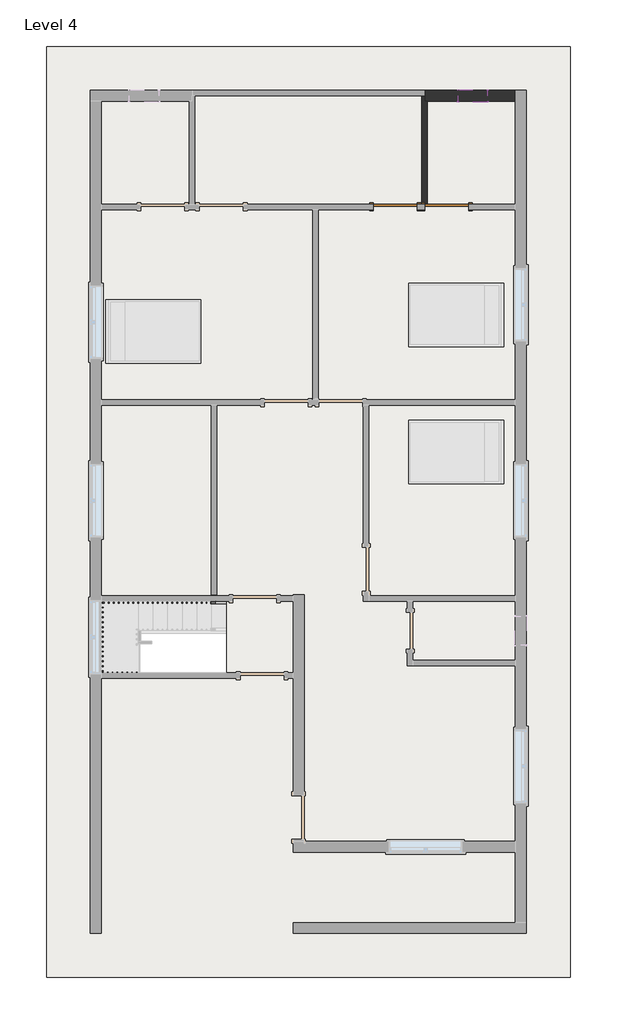
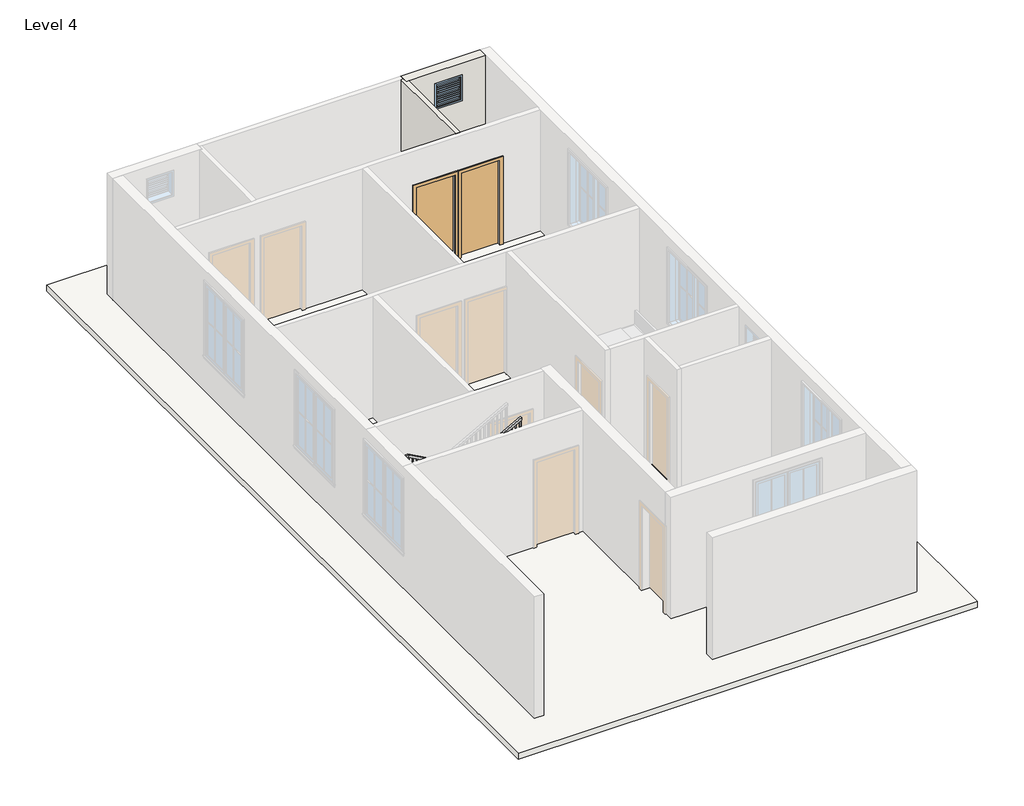
# One storey, part 2 of 3: 2 doors, 2 walls, 1 railing, 1 roof, 1 window.
"""IFC4 building model written with IfcOpenShell, lengths in millimetres."""

from ifc_helpers import new_model, si_unit, frame, origin, place, context, project, spatial, polyline, outline, extrude, faceted_brep, transform, mapped, element, save
from components import single_flush_door_3_e5f9f3c4, single_flush_door_3_305aa2a5, window_f2d8fef0

model = new_model("IFC4")

# Units and contexts
model_context = context("Model", 3, world=origin())
ifc_project = project(units=[si_unit("LENGTHUNIT", "METRE", prefix="MILLI")], contexts=[model_context])

# Site, building, storey
site = spatial("IfcSite", under=ifc_project)
building = spatial("IfcBuilding", under=site)
storey = spatial("IfcBuildingStorey", under=building, Name="Level 4", Elevation=6400.8)

# Doors
placement = place(None, origin())
single_flush_door_3_shape = single_flush_door_3_e5f9f3c4(model_context)
element("IfcDoor", 1, ObjectType="Single-Flush : DOOR 3'", at=placement, inside=storey, context=model_context, shape_type="MappedRepresentation", body=[
    mapped(single_flush_door_3_shape, transform((555.4379845, 6040.5434309, 6400.8), x_axis=(1.0, 0.0, 0.0), y_axis=(0.0, 1.0, 0.0), z_axis=(0.0, 0.0, 1.0))),
])
single_flush_door_3_2_shape = single_flush_door_3_305aa2a5(model_context)
element("IfcDoor", 2, ObjectType="Single-Flush : DOOR 3'", at=placement, inside=storey, context=model_context, shape_type="MappedRepresentation", body=[
    mapped(single_flush_door_3_2_shape, transform((1622.2379845, 6040.5434309, 6400.8), x_axis=(-1.0, 0.0, 0.0), y_axis=(0.0, -1.0, 0.0), z_axis=(0.0, 0.0, 1.0))),
])

# Railing
element("IfcRailing", 3, ObjectType="Handrail - Rectangular", at=placement, inside=storey, context=model_context, shape_type="SolidModel", body=[
    faceted_brep([(-2968.8120155, -2220.8065691, 7484.5333333), (-2968.8120155, -2220.8065691, 7426.420221), (-2968.8120155, -2170.0065691, 7426.420221), (-2968.8120155, -2170.0065691, 7484.5333333), (-4797.6120155, -2220.8065691, 8500.5333333), (-4810.7756177, -2220.8065691, 8449.7333333), (-4810.7756177, -2170.0065691, 8449.7333333), (-4797.6120155, -2170.0065691, 8500.5333333), (-5508.8120155, -2220.8065691, 8500.5333333), (-5508.8120155, -2220.8065691, 8449.7333333), (-5559.6120155, -2170.0065691, 8449.7333333), (-5559.6120155, -2170.0065691, 8500.5333333), (-5508.8120155, -3624.1565691, 8500.5333333), (-5508.8120155, -3624.1565691, 8449.7333333), (-5559.6120155, -3674.9565691, 8449.7333333), (-5559.6120155, -3674.9565691, 8500.5333333), (-5102.4120155, -3624.1565691, 8500.5333333), (-5089.2484132, -3624.1565691, 8449.7333333), (-5089.2484132, -3674.9565691, 8449.7333333), (-5102.4120155, -3674.9565691, 8500.5333333), (-2968.8120155, -3624.1565691, 9685.8666667), (-2968.8120155, -3674.9565691, 9685.8666667), (-2968.8120155, -3674.9565691, 9627.7535543), (-2968.8120155, -3624.1565691, 9627.7535543)], [[[0, 1, 2, 3]], [[1, 0, 4, 5]], [[2, 1, 5, 6]], [[3, 2, 6, 7]], [[0, 3, 7, 4]], [[5, 4, 8, 9]], [[6, 5, 9, 10]], [[7, 6, 10, 11]], [[4, 7, 11, 8]], [[9, 8, 12, 13]], [[10, 9, 13, 14]], [[11, 10, 14, 15]], [[8, 11, 15, 12]], [[13, 12, 16, 17]], [[14, 13, 17, 18]], [[15, 14, 18, 19]], [[12, 15, 19, 16]], [[20, 21, 22, 23]], [[17, 16, 20, 23]], [[18, 17, 23, 22]], [[19, 18, 22, 21]], [[16, 19, 21, 20]]]),
    extrude(outline(polyline([(9618.9341099, -2984.6870155), (9608.3507765, -3003.7370155), (8602.1333333, -3003.7370155), (8602.1333333, -2984.6870155), (9618.9341099, -2984.6870155)])), frame((0.0, -3659.0815691, 0.0), z_axis=(0.0, 1.0, 0.0), x_axis=(0.0, 0.0, 1.0)), (0.0, 0.0, 1.0), 19.05),
    extrude(outline(polyline([(9562.4896654, -3086.2870155), (9551.9063321, -3105.3370155), (8602.1333333, -3105.3370155), (8602.1333333, -3086.2870155), (9562.4896654, -3086.2870155)])), frame((0.0, -3659.0815691, 0.0), z_axis=(0.0, 1.0, 0.0), x_axis=(0.0, 0.0, 1.0)), (0.0, 0.0, 1.0), 19.05),
    extrude(outline(polyline([(9506.045221, -3187.8870155), (9495.4618876, -3206.9370155), (8602.1333333, -3206.9370155), (8602.1333333, -3187.8870155), (9506.045221, -3187.8870155)])), frame((0.0, -3659.0815691, 0.0), z_axis=(0.0, 1.0, 0.0), x_axis=(0.0, 0.0, 1.0)), (0.0, 0.0, 1.0), 19.05),
    extrude(outline(polyline([(9449.6007765, -3289.4870155), (9439.0174432, -3308.5370155), (8432.8, -3308.5370155), (8432.8, -3289.4870155), (9449.6007765, -3289.4870155)])), frame((0.0, -3659.0815691, 0.0), z_axis=(0.0, 1.0, 0.0), x_axis=(0.0, 0.0, 1.0)), (0.0, 0.0, 1.0), 19.05),
    extrude(outline(polyline([(9393.1563321, -3391.0870155), (9382.5729988, -3410.1370155), (8432.8, -3410.1370155), (8432.8, -3391.0870155), (9393.1563321, -3391.0870155)])), frame((0.0, -3659.0815691, 0.0), z_axis=(0.0, 1.0, 0.0), x_axis=(0.0, 0.0, 1.0)), (0.0, 0.0, 1.0), 19.05),
    extrude(outline(polyline([(9336.7118876, -3492.6870155), (9326.1285543, -3511.7370155), (8432.8, -3511.7370155), (8432.8, -3492.6870155), (9336.7118876, -3492.6870155)])), frame((0.0, -3659.0815691, 0.0), z_axis=(0.0, 1.0, 0.0), x_axis=(0.0, 0.0, 1.0)), (0.0, 0.0, 1.0), 19.05),
    extrude(outline(polyline([(9280.2674432, -3594.2870155), (9269.6841099, -3613.3370155), (8263.4666667, -3613.3370155), (8263.4666667, -3594.2870155), (9280.2674432, -3594.2870155)])), frame((0.0, -3659.0815691, 0.0), z_axis=(0.0, 1.0, 0.0), x_axis=(0.0, 0.0, 1.0)), (0.0, 0.0, 1.0), 19.05),
    extrude(outline(polyline([(9223.8229988, -3695.8870155), (9213.2396654, -3714.9370155), (8263.4666667, -3714.9370155), (8263.4666667, -3695.8870155), (9223.8229988, -3695.8870155)])), frame((0.0, -3659.0815691, 0.0), z_axis=(0.0, 1.0, 0.0), x_axis=(0.0, 0.0, 1.0)), (0.0, 0.0, 1.0), 19.05),
    extrude(outline(polyline([(9167.3785543, -3797.4870155), (9156.795221, -3816.5370155), (8263.4666667, -3816.5370155), (8263.4666667, -3797.4870155), (9167.3785543, -3797.4870155)])), frame((0.0, -3659.0815691, 0.0), z_axis=(0.0, 1.0, 0.0), x_axis=(0.0, 0.0, 1.0)), (0.0, 0.0, 1.0), 19.05),
    extrude(outline(polyline([(9110.9341099, -3899.0870155), (9100.3507765, -3918.1370155), (8094.1333333, -3918.1370155), (8094.1333333, -3899.0870155), (9110.9341099, -3899.0870155)])), frame((0.0, -3659.0815691, 0.0), z_axis=(0.0, 1.0, 0.0), x_axis=(0.0, 0.0, 1.0)), (0.0, 0.0, 1.0), 19.05),
    extrude(outline(polyline([(9054.4896654, -4000.6870155), (9043.9063321, -4019.7370155), (8094.1333333, -4019.7370155), (8094.1333333, -4000.6870155), (9054.4896654, -4000.6870155)])), frame((0.0, -3659.0815691, 0.0), z_axis=(0.0, 1.0, 0.0), x_axis=(0.0, 0.0, 1.0)), (0.0, 0.0, 1.0), 19.05),
    extrude(outline(polyline([(8998.045221, -4102.2870155), (8987.4618876, -4121.3370155), (8094.1333333, -4121.3370155), (8094.1333333, -4102.2870155), (8998.045221, -4102.2870155)])), frame((0.0, -3659.0815691, 0.0), z_axis=(0.0, 1.0, 0.0), x_axis=(0.0, 0.0, 1.0)), (0.0, 0.0, 1.0), 19.05),
    extrude(outline(polyline([(8941.6007765, -4203.8870155), (8931.0174432, -4222.9370155), (7924.8, -4222.9370155), (7924.8, -4203.8870155), (8941.6007765, -4203.8870155)])), frame((0.0, -3659.0815691, 0.0), z_axis=(0.0, 1.0, 0.0), x_axis=(0.0, 0.0, 1.0)), (0.0, 0.0, 1.0), 19.05),
    extrude(outline(polyline([(8885.1563321, -4305.4870155), (8874.5729988, -4324.5370155), (7924.8, -4324.5370155), (7924.8, -4305.4870155), (8885.1563321, -4305.4870155)])), frame((0.0, -3659.0815691, 0.0), z_axis=(0.0, 1.0, 0.0), x_axis=(0.0, 0.0, 1.0)), (0.0, 0.0, 1.0), 19.05),
    extrude(outline(polyline([(8828.7118876, -4407.0870155), (8818.1285543, -4426.1370155), (7924.8, -4426.1370155), (7924.8, -4407.0870155), (8828.7118876, -4407.0870155)])), frame((0.0, -3659.0815691, 0.0), z_axis=(0.0, 1.0, 0.0), x_axis=(0.0, 0.0, 1.0)), (0.0, 0.0, 1.0), 19.05),
    extrude(outline(polyline([(8772.2674432, -4508.6870155), (8761.6841099, -4527.7370155), (7755.4666667, -4527.7370155), (7755.4666667, -4508.6870155), (8772.2674432, -4508.6870155)])), frame((0.0, -3659.0815691, 0.0), z_axis=(0.0, 1.0, 0.0), x_axis=(0.0, 0.0, 1.0)), (0.0, 0.0, 1.0), 19.05),
    extrude(outline(polyline([(8715.8229988, -4610.2870155), (8705.2396654, -4629.3370155), (7755.4666667, -4629.3370155), (7755.4666667, -4610.2870155), (8715.8229988, -4610.2870155)])), frame((0.0, -3659.0815691, 0.0), z_axis=(0.0, 1.0, 0.0), x_axis=(0.0, 0.0, 1.0)), (0.0, 0.0, 1.0), 19.05),
    extrude(outline(polyline([(8659.3785543, -4711.8870155), (8648.795221, -4730.9370155), (7755.4666667, -4730.9370155), (7755.4666667, -4711.8870155), (8659.3785543, -4711.8870155)])), frame((0.0, -3659.0815691, 0.0), z_axis=(0.0, 1.0, 0.0), x_axis=(0.0, 0.0, 1.0)), (0.0, 0.0, 1.0), 19.05),
    extrude(outline(polyline([(8602.9341099, -4813.4870155), (8592.3507765, -4832.5370155), (7586.1333333, -4832.5370155), (7586.1333333, -4813.4870155), (8602.9341099, -4813.4870155)])), frame((0.0, -3659.0815691, 0.0), z_axis=(0.0, 1.0, 0.0), x_axis=(0.0, 0.0, 1.0)), (0.0, 0.0, 1.0), 19.05),
    extrude(outline(polyline([(8546.4896654, -4915.0870155), (8535.9063321, -4934.1370155), (7586.1333333, -4934.1370155), (7586.1333333, -4915.0870155), (8546.4896654, -4915.0870155)])), frame((0.0, -3659.0815691, 0.0), z_axis=(0.0, 1.0, 0.0), x_axis=(0.0, 0.0, 1.0)), (0.0, 0.0, 1.0), 19.05),
    extrude(outline(polyline([(8490.045221, -5016.6870155), (8479.4618876, -5035.7370155), (7586.1333333, -5035.7370155), (7586.1333333, -5016.6870155), (8490.045221, -5016.6870155)])), frame((0.0, -3659.0815691, 0.0), z_axis=(0.0, 1.0, 0.0), x_axis=(0.0, 0.0, 1.0)), (0.0, 0.0, 1.0), 19.05),
    extrude(outline(polyline([(-5137.3370155, -3659.0815691), (-5137.3370155, -3640.0315691), (-5118.2870155, -3640.0315691), (-5118.2870155, -3659.0815691), (-5137.3370155, -3659.0815691)])), frame((0.0, 0.0, 7586.1333333), z_axis=(0.0, 0.0, 1.0), x_axis=(1.0, 0.0, 0.0)), (0.0, 0.0, 1.0), 863.6),
    extrude(outline(polyline([(-5238.9370155, -3659.0815691), (-5238.9370155, -3640.0315691), (-5219.8870155, -3640.0315691), (-5219.8870155, -3659.0815691), (-5238.9370155, -3659.0815691)])), frame((0.0, 0.0, 7586.1333333), z_axis=(0.0, 0.0, 1.0), x_axis=(1.0, 0.0, 0.0)), (0.0, 0.0, 1.0), 863.6),
    extrude(outline(polyline([(-5340.5370155, -3659.0815691), (-5340.5370155, -3640.0315691), (-5321.4870155, -3640.0315691), (-5321.4870155, -3659.0815691), (-5340.5370155, -3659.0815691)])), frame((0.0, 0.0, 7586.1333333), z_axis=(0.0, 0.0, 1.0), x_axis=(1.0, 0.0, 0.0)), (0.0, 0.0, 1.0), 863.6),
    extrude(outline(polyline([(-5442.1370155, -3659.0815691), (-5442.1370155, -3640.0315691), (-5423.0870155, -3640.0315691), (-5423.0870155, -3659.0815691), (-5442.1370155, -3659.0815691)])), frame((0.0, 0.0, 7586.1333333), z_axis=(0.0, 0.0, 1.0), x_axis=(1.0, 0.0, 0.0)), (0.0, 0.0, 1.0), 863.6),
    extrude(outline(polyline([(-5543.7370155, -3608.2815691), (-5524.6870155, -3608.2815691), (-5524.6870155, -3627.3315691), (-5543.7370155, -3627.3315691), (-5543.7370155, -3608.2815691)])), frame((0.0, 0.0, 7586.1333333), z_axis=(0.0, 0.0, 1.0), x_axis=(1.0, 0.0, 0.0)), (0.0, 0.0, 1.0), 863.6),
    extrude(outline(polyline([(-5543.7370155, -3506.6815691), (-5524.6870155, -3506.6815691), (-5524.6870155, -3525.7315691), (-5543.7370155, -3525.7315691), (-5543.7370155, -3506.6815691)])), frame((0.0, 0.0, 7586.1333333), z_axis=(0.0, 0.0, 1.0), x_axis=(1.0, 0.0, 0.0)), (0.0, 0.0, 1.0), 863.6),
    extrude(outline(polyline([(-5543.7370155, -3405.0815691), (-5524.6870155, -3405.0815691), (-5524.6870155, -3424.1315691), (-5543.7370155, -3424.1315691), (-5543.7370155, -3405.0815691)])), frame((0.0, 0.0, 7586.1333333), z_axis=(0.0, 0.0, 1.0), x_axis=(1.0, 0.0, 0.0)), (0.0, 0.0, 1.0), 863.6),
    extrude(outline(polyline([(-5543.7370155, -3303.4815691), (-5524.6870155, -3303.4815691), (-5524.6870155, -3322.5315691), (-5543.7370155, -3322.5315691), (-5543.7370155, -3303.4815691)])), frame((0.0, 0.0, 7586.1333333), z_axis=(0.0, 0.0, 1.0), x_axis=(1.0, 0.0, 0.0)), (0.0, 0.0, 1.0), 863.6),
    extrude(outline(polyline([(-5543.7370155, -3201.8815691), (-5524.6870155, -3201.8815691), (-5524.6870155, -3220.9315691), (-5543.7370155, -3220.9315691), (-5543.7370155, -3201.8815691)])), frame((0.0, 0.0, 7586.1333333), z_axis=(0.0, 0.0, 1.0), x_axis=(1.0, 0.0, 0.0)), (0.0, 0.0, 1.0), 863.6),
    extrude(outline(polyline([(-5543.7370155, -3100.2815691), (-5524.6870155, -3100.2815691), (-5524.6870155, -3119.3315691), (-5543.7370155, -3119.3315691), (-5543.7370155, -3100.2815691)])), frame((0.0, 0.0, 7586.1333333), z_axis=(0.0, 0.0, 1.0), x_axis=(1.0, 0.0, 0.0)), (0.0, 0.0, 1.0), 863.6),
    extrude(outline(polyline([(-5543.7370155, -2998.6815691), (-5524.6870155, -2998.6815691), (-5524.6870155, -3017.7315691), (-5543.7370155, -3017.7315691), (-5543.7370155, -2998.6815691)])), frame((0.0, 0.0, 7586.1333333), z_axis=(0.0, 0.0, 1.0), x_axis=(1.0, 0.0, 0.0)), (0.0, 0.0, 1.0), 863.6),
    extrude(outline(polyline([(-5543.7370155, -2897.0815691), (-5524.6870155, -2897.0815691), (-5524.6870155, -2916.1315691), (-5543.7370155, -2916.1315691), (-5543.7370155, -2897.0815691)])), frame((0.0, 0.0, 7586.1333333), z_axis=(0.0, 0.0, 1.0), x_axis=(1.0, 0.0, 0.0)), (0.0, 0.0, 1.0), 863.6),
    extrude(outline(polyline([(-5543.7370155, -2795.4815691), (-5524.6870155, -2795.4815691), (-5524.6870155, -2814.5315691), (-5543.7370155, -2814.5315691), (-5543.7370155, -2795.4815691)])), frame((0.0, 0.0, 7586.1333333), z_axis=(0.0, 0.0, 1.0), x_axis=(1.0, 0.0, 0.0)), (0.0, 0.0, 1.0), 863.6),
    extrude(outline(polyline([(-5543.7370155, -2693.8815691), (-5524.6870155, -2693.8815691), (-5524.6870155, -2712.9315691), (-5543.7370155, -2712.9315691), (-5543.7370155, -2693.8815691)])), frame((0.0, 0.0, 7586.1333333), z_axis=(0.0, 0.0, 1.0), x_axis=(1.0, 0.0, 0.0)), (0.0, 0.0, 1.0), 863.6),
    extrude(outline(polyline([(-5543.7370155, -2592.2815691), (-5524.6870155, -2592.2815691), (-5524.6870155, -2611.3315691), (-5543.7370155, -2611.3315691), (-5543.7370155, -2592.2815691)])), frame((0.0, 0.0, 7586.1333333), z_axis=(0.0, 0.0, 1.0), x_axis=(1.0, 0.0, 0.0)), (0.0, 0.0, 1.0), 863.6),
    extrude(outline(polyline([(-5543.7370155, -2490.6815691), (-5524.6870155, -2490.6815691), (-5524.6870155, -2509.7315691), (-5543.7370155, -2509.7315691), (-5543.7370155, -2490.6815691)])), frame((0.0, 0.0, 7586.1333333), z_axis=(0.0, 0.0, 1.0), x_axis=(1.0, 0.0, 0.0)), (0.0, 0.0, 1.0), 863.6),
    extrude(outline(polyline([(-5543.7370155, -2389.0815691), (-5524.6870155, -2389.0815691), (-5524.6870155, -2408.1315691), (-5543.7370155, -2408.1315691), (-5543.7370155, -2389.0815691)])), frame((0.0, 0.0, 7586.1333333), z_axis=(0.0, 0.0, 1.0), x_axis=(1.0, 0.0, 0.0)), (0.0, 0.0, 1.0), 863.6),
    extrude(outline(polyline([(-5543.7370155, -2287.4815691), (-5524.6870155, -2287.4815691), (-5524.6870155, -2306.5315691), (-5543.7370155, -2306.5315691), (-5543.7370155, -2287.4815691)])), frame((0.0, 0.0, 7586.1333333), z_axis=(0.0, 0.0, 1.0), x_axis=(1.0, 0.0, 0.0)), (0.0, 0.0, 1.0), 863.6),
    extrude(outline(polyline([(-5499.2870155, -2185.8815691), (-5499.2870155, -2204.9315691), (-5518.3370155, -2204.9315691), (-5518.3370155, -2185.8815691), (-5499.2870155, -2185.8815691)])), frame((0.0, 0.0, 7586.1333333), z_axis=(0.0, 0.0, 1.0), x_axis=(1.0, 0.0, 0.0)), (0.0, 0.0, 1.0), 863.6),
    extrude(outline(polyline([(-5397.6870155, -2185.8815691), (-5397.6870155, -2204.9315691), (-5416.7370155, -2204.9315691), (-5416.7370155, -2185.8815691), (-5397.6870155, -2185.8815691)])), frame((0.0, 0.0, 7586.1333333), z_axis=(0.0, 0.0, 1.0), x_axis=(1.0, 0.0, 0.0)), (0.0, 0.0, 1.0), 863.6),
    extrude(outline(polyline([(-5296.0870155, -2185.8815691), (-5296.0870155, -2204.9315691), (-5315.1370155, -2204.9315691), (-5315.1370155, -2185.8815691), (-5296.0870155, -2185.8815691)])), frame((0.0, 0.0, 7586.1333333), z_axis=(0.0, 0.0, 1.0), x_axis=(1.0, 0.0, 0.0)), (0.0, 0.0, 1.0), 863.6),
    extrude(outline(polyline([(-5194.4870155, -2185.8815691), (-5194.4870155, -2204.9315691), (-5213.5370155, -2204.9315691), (-5213.5370155, -2185.8815691), (-5194.4870155, -2185.8815691)])), frame((0.0, 0.0, 7586.1333333), z_axis=(0.0, 0.0, 1.0), x_axis=(1.0, 0.0, 0.0)), (0.0, 0.0, 1.0), 863.6),
    extrude(outline(polyline([(-5092.8870155, -2185.8815691), (-5092.8870155, -2204.9315691), (-5111.9370155, -2204.9315691), (-5111.9370155, -2185.8815691), (-5092.8870155, -2185.8815691)])), frame((0.0, 0.0, 7586.1333333), z_axis=(0.0, 0.0, 1.0), x_axis=(1.0, 0.0, 0.0)), (0.0, 0.0, 1.0), 863.6),
    extrude(outline(polyline([(-4991.2870155, -2185.8815691), (-4991.2870155, -2204.9315691), (-5010.3370155, -2204.9315691), (-5010.3370155, -2185.8815691), (-4991.2870155, -2185.8815691)])), frame((0.0, 0.0, 7586.1333333), z_axis=(0.0, 0.0, 1.0), x_axis=(1.0, 0.0, 0.0)), (0.0, 0.0, 1.0), 863.6),
    extrude(outline(polyline([(-4889.6870155, -2185.8815691), (-4889.6870155, -2204.9315691), (-4908.7370155, -2204.9315691), (-4908.7370155, -2185.8815691), (-4889.6870155, -2185.8815691)])), frame((0.0, 0.0, 7586.1333333), z_axis=(0.0, 0.0, 1.0), x_axis=(1.0, 0.0, 0.0)), (0.0, 0.0, 1.0), 863.6),
    extrude(outline(polyline([(8437.1285543, -4788.0870155), (8447.7118876, -4807.1370155), (7586.1333333, -4807.1370155), (7586.1333333, -4788.0870155), (8437.1285543, -4788.0870155)])), frame((0.0, -2204.9315691, 0.0), z_axis=(0.0, 1.0, 0.0), x_axis=(0.0, 0.0, 1.0)), (0.0, 0.0, 1.0), 19.05),
    extrude(outline(polyline([(8380.6841099, -4686.4870155), (8391.2674432, -4705.5370155), (7416.8, -4705.5370155), (7416.8, -4686.4870155), (8380.6841099, -4686.4870155)])), frame((0.0, -2204.9315691, 0.0), z_axis=(0.0, 1.0, 0.0), x_axis=(0.0, 0.0, 1.0)), (0.0, 0.0, 1.0), 19.05),
    extrude(outline(polyline([(8324.2396654, -4584.8870155), (8334.8229988, -4603.9370155), (7416.8, -4603.9370155), (7416.8, -4584.8870155), (8324.2396654, -4584.8870155)])), frame((0.0, -2204.9315691, 0.0), z_axis=(0.0, 1.0, 0.0), x_axis=(0.0, 0.0, 1.0)), (0.0, 0.0, 1.0), 19.05),
    extrude(outline(polyline([(8267.795221, -4483.2870155), (8278.3785543, -4502.3370155), (7416.8, -4502.3370155), (7416.8, -4483.2870155), (8267.795221, -4483.2870155)])), frame((0.0, -2204.9315691, 0.0), z_axis=(0.0, 1.0, 0.0), x_axis=(0.0, 0.0, 1.0)), (0.0, 0.0, 1.0), 19.05),
    extrude(outline(polyline([(8211.3507765, -4381.6870155), (8221.9341099, -4400.7370155), (7247.4666667, -4400.7370155), (7247.4666667, -4381.6870155), (8211.3507765, -4381.6870155)])), frame((0.0, -2204.9315691, 0.0), z_axis=(0.0, 1.0, 0.0), x_axis=(0.0, 0.0, 1.0)), (0.0, 0.0, 1.0), 19.05),
    extrude(outline(polyline([(8154.9063321, -4280.0870155), (8165.4896654, -4299.1370155), (7247.4666667, -4299.1370155), (7247.4666667, -4280.0870155), (8154.9063321, -4280.0870155)])), frame((0.0, -2204.9315691, 0.0), z_axis=(0.0, 1.0, 0.0), x_axis=(0.0, 0.0, 1.0)), (0.0, 0.0, 1.0), 19.05),
    extrude(outline(polyline([(8098.4618876, -4178.4870155), (8109.045221, -4197.5370155), (7247.4666667, -4197.5370155), (7247.4666667, -4178.4870155), (8098.4618876, -4178.4870155)])), frame((0.0, -2204.9315691, 0.0), z_axis=(0.0, 1.0, 0.0), x_axis=(0.0, 0.0, 1.0)), (0.0, 0.0, 1.0), 19.05),
    extrude(outline(polyline([(8042.0174432, -4076.8870155), (8052.6007765, -4095.9370155), (7078.1333333, -4095.9370155), (7078.1333333, -4076.8870155), (8042.0174432, -4076.8870155)])), frame((0.0, -2204.9315691, 0.0), z_axis=(0.0, 1.0, 0.0), x_axis=(0.0, 0.0, 1.0)), (0.0, 0.0, 1.0), 19.05),
    extrude(outline(polyline([(7985.5729988, -3975.2870155), (7996.1563321, -3994.3370155), (7078.1333333, -3994.3370155), (7078.1333333, -3975.2870155), (7985.5729988, -3975.2870155)])), frame((0.0, -2204.9315691, 0.0), z_axis=(0.0, 1.0, 0.0), x_axis=(0.0, 0.0, 1.0)), (0.0, 0.0, 1.0), 19.05),
    extrude(outline(polyline([(7929.1285543, -3873.6870155), (7939.7118876, -3892.7370155), (7078.1333333, -3892.7370155), (7078.1333333, -3873.6870155), (7929.1285543, -3873.6870155)])), frame((0.0, -2204.9315691, 0.0), z_axis=(0.0, 1.0, 0.0), x_axis=(0.0, 0.0, 1.0)), (0.0, 0.0, 1.0), 19.05),
    extrude(outline(polyline([(7872.6841099, -3772.0870155), (7883.2674432, -3791.1370155), (6908.8, -3791.1370155), (6908.8, -3772.0870155), (7872.6841099, -3772.0870155)])), frame((0.0, -2204.9315691, 0.0), z_axis=(0.0, 1.0, 0.0), x_axis=(0.0, 0.0, 1.0)), (0.0, 0.0, 1.0), 19.05),
    extrude(outline(polyline([(7816.2396654, -3670.4870155), (7826.8229988, -3689.5370155), (6908.8, -3689.5370155), (6908.8, -3670.4870155), (7816.2396654, -3670.4870155)])), frame((0.0, -2204.9315691, 0.0), z_axis=(0.0, 1.0, 0.0), x_axis=(0.0, 0.0, 1.0)), (0.0, 0.0, 1.0), 19.05),
    extrude(outline(polyline([(7759.795221, -3568.8870155), (7770.3785543, -3587.9370155), (6908.8, -3587.9370155), (6908.8, -3568.8870155), (7759.795221, -3568.8870155)])), frame((0.0, -2204.9315691, 0.0), z_axis=(0.0, 1.0, 0.0), x_axis=(0.0, 0.0, 1.0)), (0.0, 0.0, 1.0), 19.05),
    extrude(outline(polyline([(7703.3507765, -3467.2870155), (7713.9341099, -3486.3370155), (6739.4666667, -3486.3370155), (6739.4666667, -3467.2870155), (7703.3507765, -3467.2870155)])), frame((0.0, -2204.9315691, 0.0), z_axis=(0.0, 1.0, 0.0), x_axis=(0.0, 0.0, 1.0)), (0.0, 0.0, 1.0), 19.05),
    extrude(outline(polyline([(7646.9063321, -3365.6870155), (7657.4896654, -3384.7370155), (6739.4666667, -3384.7370155), (6739.4666667, -3365.6870155), (7646.9063321, -3365.6870155)])), frame((0.0, -2204.9315691, 0.0), z_axis=(0.0, 1.0, 0.0), x_axis=(0.0, 0.0, 1.0)), (0.0, 0.0, 1.0), 19.05),
    extrude(outline(polyline([(7590.4618876, -3264.0870155), (7601.045221, -3283.1370155), (6739.4666667, -3283.1370155), (6739.4666667, -3264.0870155), (7590.4618876, -3264.0870155)])), frame((0.0, -2204.9315691, 0.0), z_axis=(0.0, 1.0, 0.0), x_axis=(0.0, 0.0, 1.0)), (0.0, 0.0, 1.0), 19.05),
    extrude(outline(polyline([(7534.0174432, -3162.4870155), (7544.6007765, -3181.5370155), (6570.1333333, -3181.5370155), (6570.1333333, -3162.4870155), (7534.0174432, -3162.4870155)])), frame((0.0, -2204.9315691, 0.0), z_axis=(0.0, 1.0, 0.0), x_axis=(0.0, 0.0, 1.0)), (0.0, 0.0, 1.0), 19.05),
    extrude(outline(polyline([(7477.5729988, -3060.8870155), (7488.1563321, -3079.9370155), (6570.1333333, -3079.9370155), (6570.1333333, -3060.8870155), (7477.5729988, -3060.8870155)])), frame((0.0, -2204.9315691, 0.0), z_axis=(0.0, 1.0, 0.0), x_axis=(0.0, 0.0, 1.0)), (0.0, 0.0, 1.0), 19.05),
    extrude(outline(polyline([(-5543.7370155, -3640.0315691), (-5524.6870155, -3640.0315691), (-5524.6870155, -3659.0815691), (-5543.7370155, -3659.0815691), (-5543.7370155, -3640.0315691)])), frame((0.0, 0.0, 7586.1333333), z_axis=(0.0, 0.0, 1.0), x_axis=(1.0, 0.0, 0.0)), (0.0, 0.0, 1.0), 863.6),
    extrude(outline(polyline([(-5524.6870155, -2185.8815691), (-5524.6870155, -2204.9315691), (-5543.7370155, -2204.9315691), (-5543.7370155, -2185.8815691), (-5524.6870155, -2185.8815691)])), frame((0.0, 0.0, 7586.1333333), z_axis=(0.0, 0.0, 1.0), x_axis=(1.0, 0.0, 0.0)), (0.0, 0.0, 1.0), 863.6),
    extrude(outline(polyline([(9627.7535543, -2968.8120155), (9617.170221, -2987.8620155), (8602.1333333, -2987.8620155), (8602.1333333, -2968.8120155), (9627.7535543, -2968.8120155)])), frame((0.0, -3659.0815691, 0.0), z_axis=(0.0, 1.0, 0.0), x_axis=(0.0, 0.0, 1.0)), (0.0, 0.0, 1.0), 19.05),
    extrude(outline(polyline([(7426.420221, -2968.8120155), (7437.0035543, -2987.8620155), (6570.1333333, -2987.8620155), (6570.1333333, -2968.8120155), (7426.420221, -2968.8120155)])), frame((0.0, -2204.9315691, 0.0), z_axis=(0.0, 1.0, 0.0), x_axis=(0.0, 0.0, 1.0)), (0.0, 0.0, 1.0), 19.05),
])

# Roof
element("IfcRoof", 4, ObjectType="ROOF 6\"", at=placement, inside=storey, context=model_context, shape_type="SweptSolid", body=[
    extrude(outline(polyline([(4193.9879845, 9374.2934309), (4193.9879845, -9993.2065691), (-6702.6120155, -9993.2065691), (-6702.6120155, 9374.2934309), (4193.9879845, 9374.2934309)]), holes=[polyline([(-2968.8120155, -2150.9565691), (-5788.2120155, -2150.9565691), (-5788.2120155, -3674.9565691), (-2968.8120155, -3674.9565691), (-2968.8120155, -2150.9565691)])]), frame((0.0, 0.0, 6248.4), z_axis=(0.0, 0.0, 1.0), x_axis=(1.0, 0.0, 0.0)), (0.0, 0.0, 1.0), 152.4),
])

# Walls
element("IfcWall", 5, ObjectType="WALL 4.5\"", at=placement, inside=storey, context=model_context, shape_type="SweptSolid", body=[
    extrude(outline(polyline([(1107.8879845, 6097.6934309), (1107.8879845, 8345.5934309), (1165.0379845, 8345.5934309), (1165.0379845, 8231.2934309), (1222.1879845, 8231.2934309), (1222.1879845, 6097.6934309), (1107.8879845, 6097.6934309)])), frame((0.0, 0.0, 6400.8), z_axis=(0.0, 0.0, 1.0), x_axis=(1.0, 0.0, 0.0)), (0.0, 0.0, 1.0), 3048.0),
])
element("IfcWall", 6, ObjectType="WALL 9\"", at=placement, inside=storey, context=model_context, shape_type="Brep", body=[
    faceted_brep([(3050.9879845, 8459.8934309, 6400.8), (1165.0379845, 8459.8934309, 6400.8), (1165.0379845, 8459.8934309, 9448.8), (3050.9879845, 8459.8934309, 9448.8), (2469.9629845, 8459.8934309, 9144.0), (1860.3629845, 8459.8934309, 9144.0), (1860.3629845, 8459.8934309, 8534.4), (2469.9629845, 8459.8934309, 8534.4), (3050.9879845, 8231.2934309, 6400.8), (3050.9879845, 8231.2934309, 9448.8), (1222.1879845, 8231.2934309, 9448.8), (1165.0379845, 8231.2934309, 9448.8), (1165.0379845, 8231.2934309, 6400.8), (1222.1879845, 8231.2934309, 6400.8), (2469.9629845, 8231.2934309, 9144.0), (2469.9629845, 8231.2934309, 8534.4), (1860.3629845, 8231.2934309, 8534.4), (1860.3629845, 8231.2934309, 9144.0), (1165.0379845, 8345.5934309, 6400.8), (1165.0379845, 8345.5934309, 9448.8)], [[[0, 1, 2, 3], [4, 5, 6, 7]], [[8, 9, 10, 11, 12, 13], [14, 15, 16, 17]], [[1, 0, 8, 13, 12, 18]], [[2, 1, 18, 12, 11, 19]], [[0, 3, 9, 8]], [[15, 14, 4, 7]], [[16, 15, 7, 6]], [[17, 16, 6, 5]], [[14, 17, 5, 4]], [[3, 2, 19, 11, 10, 9]]]),
])

# Window
window_shape = window_f2d8fef0(model_context)
element("IfcWindow", 7, ObjectType="Window-Louvers : 24\" x 24\"", at=placement, inside=storey, context=model_context, shape_type="MappedRepresentation", body=[
    mapped(window_shape, transform((2165.1629845, 8339.2434309, 7620.0), x_axis=(-1.0, 0.0, 0.0), y_axis=(0.0, -1.0, 0.0), z_axis=(0.0, 0.0, 1.0))),
])

save(model, "model.ifc")

# Revit data of these elements
# Type "Single-Flush : DOOR 3'"
#   Type Mark = "9"
#   Construction Type Id = "MDOOR"
#   Assembly Code = "C1020"
#   Analytic Construction = "Metal"
#   Thickness = 0' - 2"
#   Heat Transfer Coefficient (U) = 0.651978 BTU/(h·ft²·°F)
#   Height = 7' - 0"
#   Trim Projection Ext = 0' - 1"
#   Trim Projection Int = 0' - 1"
#   Trim Width = 0' - 3"
#   Width = 3' - 0"
#   Define Thermal Properties by = 1
#   Door Material = Door - Panel
#   Frame Material = Door - Frame
#   Visual Light Transmittance = 0
#   Solar Heat Gain Coefficient = 0
#   Function = (empty or 0)
#   Wall Closure = (empty or 0)
# Type "Handrail - Rectangular"
#   Assembly Code = "C2010400"
#   built-in parameter 1008612 = 0.0416667 (stored number, unit not read)
#   built-in parameter 1008611 = 0.0416667 (stored number, unit not read)
#   built-in parameter 1008609 = 0.333333 (stored number, unit not read)
#   built-in parameter 1008604 = 0.166667 (stored number, unit not read)
#   built-in parameter 1008603 = 0.166667 (stored number, unit not read)
#   Railing Height = 3' - 0"
#   built-in parameter 1008630 = 2
#   built-in parameter 1008610 = 2
#   built-in parameter 1008618 = Baluster - Square : 3/4"
# Type "ROOF 6\""
#   Assembly Code = "B1020"
#   Layers, outside or top first: 0' - 6" no material (function 1)
# Type "WALL 4.5\""
#   Assembly Code = "B2010"
#   Layers, outside or top first: 0' - 4 1/2" no material (function 1)
# Type "WALL 9\""
#   Assembly Code = "B2010"
#   Layers, outside or top first: 0' - 9" no material (function 1)
# Type "Window-Louvers : 24\" x 24\""
#   Type Mark = "19"
#   Construction Type Id = "GSP4R"
#   Assembly Code = "B20"
#   Analytic Construction = "1/8 in Pilkington single glazing"
#   Visual Light Transmittance = 0.9
#   Thermal Resistance (R) = 1.53941 (h·ft²·°F)/BTU
#   Solar Heat Gain Coefficient = 0.78
#   Max Height = 1' - 11.74264"
#   Height = 2' - 0"
#   Heat Transfer Coefficient (U) = 0.6496 BTU/(h·ft²·°F)
#   Blade Width [instance default] = 1' - 10 1/2"
#   Blade Vertical Thickness = 0' - 0.35355"
#   Blade Thickness = 0' - 0 1/4"
#   Blade Spacing = 0' - 1 1/2"
#   Blade Height = 0' - 1.85355"
#   Blade Depth = 0' - 3"
#   Blade Angle = 45.00°
#   Default Sill Height = 3' - 0"
#   Trim Projection_Exterior = 0' - 0 1/2"
#   Trim Projection_Interior = 0' - 0 1/2"
#   Trim Width_Exterior = 0' - 1 1/2"
#   Trim Width_Interior = 0' - 1 1/2"
#   Width = 2' - 0"
#   Max Blade Count = 12
#   Define Thermal Properties by = 1
#   Blade Count = 12
#   Frame Material = Birch
#   Louver Material = Birch
#   Trim Exterior Material = Birch
#   Trim Interior Material = Birch
#   Wall Closure = (empty or 0)
# Elements 1, 2 (IfcDoor, "Single-Flush : DOOR 3'")
#   Phase Created = New Construction
#   Materials on its faces: "Door - Frame", "Door - Panel"
# Element 3 (IfcRailing, "Handrail - Rectangular")
#   Phase Created = New Construction
# Element 4 (IfcRoof, "ROOF 6\"")
#   built-in parameter 1001705 = 21 (stored number, unit not read)
#   built-in parameter 1001701 = -0.5 (stored number, unit not read)
#   built-in parameter 1001710 = 33615
#   Phase Created = New Construction
#   Materials on its faces: "Default Roof", "Brick, Common", "Birch"
# Element 5 (IfcWall, "WALL 4.5\"")
#   Top Offset = 0' - 0"
#   Base Offset = 0' - 0"
#   Unconnected Height = 10' - 0"
#   wall height = 10' - 0"
#   Phase Created = New Construction
#   Base Constraint = Level 4
#   Materials on its faces: "Default Wall"
# Element 6 (IfcWall, "WALL 9\"")
#   Top Offset = 0' - 0"
#   Base Offset = 0' - 0"
#   Unconnected Height = 10' - 0"
#   wall height = 10' - 0"
#   Phase Created = New Construction
#   Base Constraint = Level 4
#   Materials on its faces: "Default Wall", "Brick, Common"
# Element 7 (IfcWindow, "Window-Louvers : 24\" x 24\"")
#   Mark = "29"
#   Blade Width = 1' - 10 1/2"
#   Phase Created = New Construction
#   Materials on its faces: "Birch"
# Materials
#   "Door - Panel": class "Wood", colour RGB 210 159 95, transparency 0, Cost = 0
#   "Door - Frame": colour RGB 118 70 51, transparency 0, Cost = 0
#   "Birch": class "Wood", colour RGB 224 178 126, transparency 0, Description = "Betula Alleghaniensis", Cost = 0
#   "Default Roof": colour RGB 88 101 114, transparency 0, Cost = 0
#   "Brick, Common": class "Masonry", colour RGB 170 98 104, transparency 0, Description = "Common brick", Cost = 0
#   "Default Wall": colour RGB 128 128 128, transparency 0, Cost = 0
